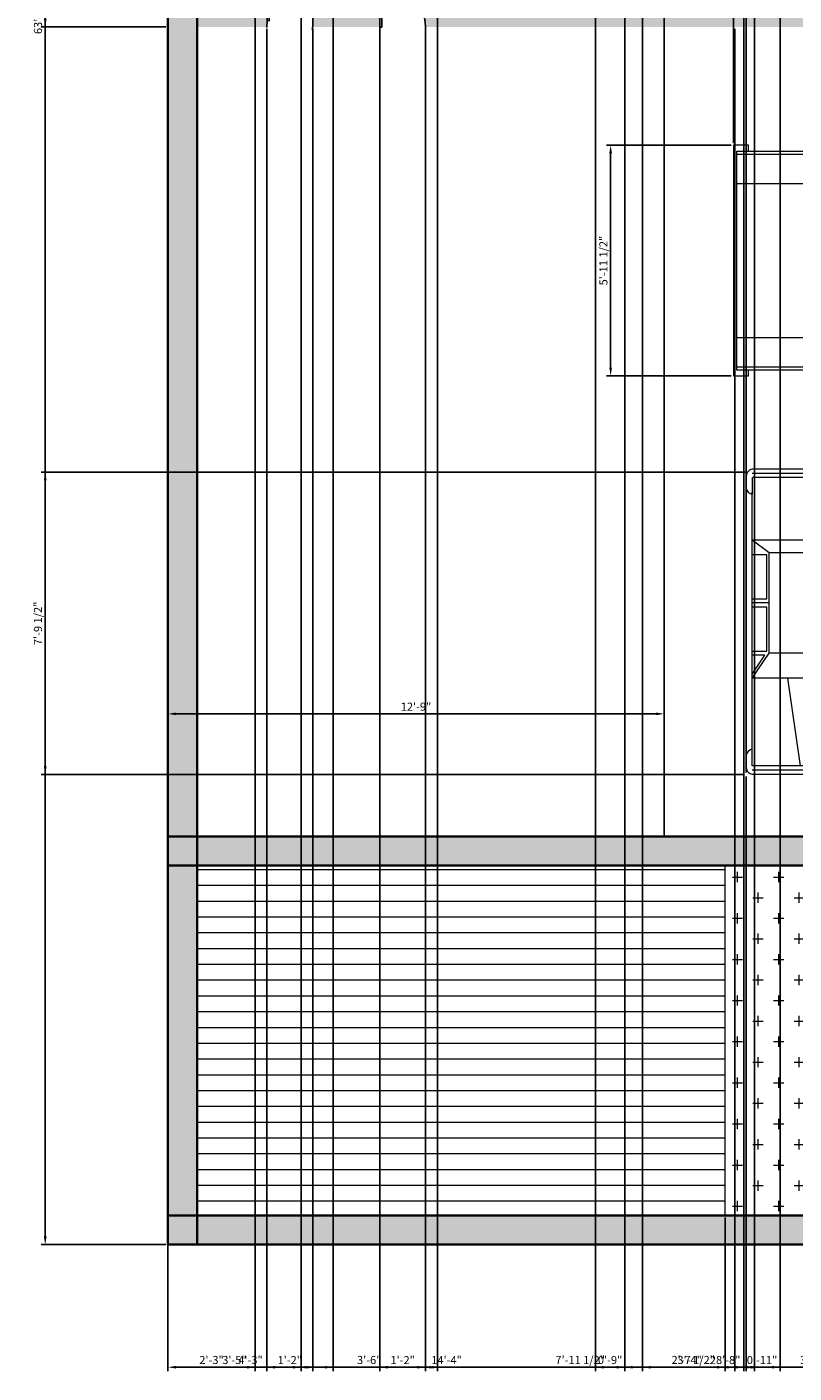
# Model space of a CAD drawing. Units: millimetres. Extents: x 2856 to 3283, y 634 to 1474.
# Tile 1 of 8: x 2856 to 3092, y 634 to 1050. Entities that reach past the tile are written whole.
import ezdxf

# ---------------------------------------------------------------- set-up
doc = ezdxf.new("R2010")
doc.units = ezdxf.units.MM
for name, color, linetype, lineweight in [('A-ANNO-DIMS', 90, 'Continuous', 18), ('A-FLOR', 50, 'Continuous', 18), ('A-FLOR-PATT', 50, 'Continuous', 13), ('A-WALL-PATT', 2, 'Continuous', 13), ('cars', 130, 'Continuous', 13), ('doors', 10, 'Continuous', 25), ('walls', 50, 'Continuous', 35)]:
    doc.layers.add(name, color=color, linetype=linetype, lineweight=lineweight)
doc.styles.get("Standard").update_dxf_attribs({"font": 'arial.ttf'})
doc.dimstyles.new('ISO-25', dxfattribs={"dimtxt": 2.5, "dimasz": 2.5, "dimexe": 1.25, "dimexo": 0.625, "dimtad": 1, "dimdec": 0, "dimlunit": 3, "dimtxsty": 'Standard', "dimcen": 2.5, "dimadec": 0, "dimazin": 0, "dimtfac": 1, "dimtdec": 0, "dimtmove": 0, "dimatfit": 3, "dimfxl": 1, "dimarcsym": 0})

# ---------------------------------------------------------------- blocks, each defined once
blk = doc.blocks.new('*U3')
for p, q in [((0, 0), (0, -6)), ((40, 0), (40, -6))]:
    blk.add_line(p, q)
blk.add_lwpolyline([(0, 0), (0, 40), (1.75, 40), (1.75, 0)], close=True)
blk.add_arc((0, 0), 40, 0, 90)
blk = doc.blocks.new('*U9')
for p, q in [((0.1, -0.41), (0.1, 38.35)), ((2.77, -0.41), (2.77, 38.31)), ((5.44, 42.31), (12.12, 42.31)), ((5.44, -0.41), (5.44, 38.24)), ((5.45, 38.31), (16.12, 38.31)), ((16.12, 38.31), (180.34, 38.31)), ((61.52, -0.41), (61.52, 38.31)), ((61.52, 38.31), (77.54, 27.62)), ((64.19, 38.31), (76.2, 30.29)), ((76.2, 30.29), (76.2, 38.31)), ((78.87, 38.31), (78.87, 28.96)), ((106.91, 28.96), (106.91, 38.31)), ((109.58, 27.62), (109.58, 38.31)), ((112.25, 38.31), (112.25, 28.96)), ((140.29, 28.96), (140.29, 38.31)), ((141.62, 27.62), (149.64, 38.31)), ((149.64, -0.41), (149.64, 38.31)), ((189.69, 38.31), (179.01, 38.31)), ((189.69, 42.31), (183.01, 42.31)), ((189.69, -0.41), (189.69, 38.24)), ((192.36, -0.41), (192.36, 38.31)), ((195.03, -0.41), (195.03, 38.35)), ((77.54, 27.62), (141.62, 27.62)), ((77.54, -0.41), (77.54, 27.62)), ((78.87, 28.96), (106.91, 28.96)), ((112.25, 28.96), (140.29, 28.96)), ((141.62, -0.41), (141.62, 27.62)), ((5.44, 7.6), (61.52, 15.61)), ((0.1, -0.42), (0.1, -39.18)), ((2.77, -0.41), (2.77, -39.13)), ((5.44, -0.42), (5.44, -39.07)), ((5.44, -8.42), (61.52, -16.43)), ((61.52, -0.41), (61.52, -39.13)), ((77.54, -0.41), (77.54, -28.45)), ((141.62, -0.41), (141.62, -28.45)), ((149.64, -0.41), (149.64, -39.13)), ((189.69, -0.42), (189.69, -39.07)), ((192.36, -0.41), (192.36, -39.13)), ((195.03, -0.42), (195.03, -39.18)), ((61.52, -39.13), (77.54, -28.45)), ((64.19, -39.13), (76.2, -31.12)), ((76.2, -31.12), (76.2, -39.13)), ((77.54, -28.45), (141.62, -28.45)), ((78.87, -39.13), (78.87, -29.79)), ((78.87, -29.79), (106.91, -29.79)), ((106.91, -29.79), (106.91, -39.13)), ((109.58, -28.45), (109.58, -39.13)), ((112.25, -29.79), (140.29, -29.79)), ((112.25, -39.13), (112.25, -29.79)), ((140.29, -29.79), (140.29, -39.13)), ((141.62, -28.45), (149.64, -39.13)), ((5.45, -39.13), (16.12, -39.13)), ((16.12, -39.13), (180.34, -39.13)), ((189.69, -39.13), (179.01, -39.13)), ((5.44, -43.14), (12.12, -43.14)), ((189.69, -43.14), (183.01, -43.14))]:
    blk.add_line(p, q)
for centre, radius, start, end in [((5.06, 37.26), 5.06, 85.64554, 168.0943), ((11.45, 37.64), 4.72, 8.13011, 81.86996), ((183.68, 37.64), 4.72, 98.13004, 171.8699), ((190.07, 37.26), 5.06, 11.90574, 94.35446), ((5.06, -38.09), 5.06, 191.9057, 274.3545), ((11.45, -38.46), 4.72, 278.13, 351.8699), ((183.68, -38.46), 4.72, 188.1301, 261.87), ((190.07, -38.09), 5.06, 265.6455, 348.0943)]:
    blk.add_arc(centre, radius, start, end)
blk = doc.blocks.new('*U10')
for p, q in [((1.28, 38.87), (175.66, 38.87)), ((1.28, 28.15), (52.13, 28.15)), ((1.28, -28.15), (52.13, -28.15)), ((1.28, -38.87), (175.66, -38.87))]:
    blk.add_line(p, q)
for points in [[(5.57, 40.01), (5.57, 42.18), (0, 42.18), (0, -42.18), (5.57, -42.18), (5.57, -40.01), (1.28, -40.01), (1.28, 40.01)], [(1.28, 40.01), (175.66, 40.01), (175.66, -40.01), (1.28, -40.01)], [(171.74, 40.01), (175.66, 40.01), (175.66, -40.01), (171.74, -40.01), (171.74, -42.18), (178.14, -42.18), (178.14, 42.18), (171.74, 42.18)], [(71.47, 21.48), (163.42, 21.48), (163.42, -21.48), (71.47, -21.48)]]:
    blk.add_lwpolyline(points, close=True)
for points in [[(57.15, 40.01), (57.15, 32.39), (71.72, 22.83, 0.086577), (72.56, 22.68), (91.59, 22.68, 0.227875), (93.54, 23.62), (97.72, 32.11), (97.72, 40.01)], [(57.15, -40.01), (57.15, -32.39), (71.72, -22.83, -0.086577), (72.56, -22.68), (91.59, -22.68, -0.227875), (93.54, -23.62), (97.72, -32.11), (97.72, -40.01)]]:
    blk.add_lwpolyline(points, format="xyb")
for points in [[(62.08, 30.95), (72.14, 24.35, 0.146139), (72.69, 24.18), (91.42, 24.18, 0.29766), (92.33, 24.78), (95.09, 31.05, 0.541236), (94.86, 31.41), (62.21, 31.41, 0.744989)], [(102.19, 24.58), (106.97, 31, -0.236929), (107.78, 31.41), (162.91, 31.41, -0.621576), (163.11, 31), (158.19, 24.58, -0.233368), (157.39, 24.18), (102.39, 24.18, -0.616908)], [(55.49, 27.42), (68.59, 20.89, -0.284287), (69.14, 19.99), (69.14, -19.99, -0.284287), (68.59, -20.89), (55.49, -27.42, -0.557284), (54.05, -26.53), (54.05, 26.53, -0.557284)], [(171.88, 27.31), (166.83, 24.47, 0.271143), (166.32, 23.6), (166.32, -23.6, 0.271143), (166.83, -24.47), (171.88, -27.31, 0.573387), (173.37, -26.44), (173.37, 26.44, 0.573387)], [(62.08, -30.95), (72.14, -24.35, -0.146139), (72.69, -24.18), (91.42, -24.18, -0.29766), (92.33, -24.78), (95.09, -31.05, -0.541236), (94.86, -31.41), (62.21, -31.41, -0.744989)], [(102.19, -24.58), (106.97, -31, 0.236929), (107.78, -31.41), (162.91, -31.41, 0.621576), (163.11, -31), (158.19, -24.58, 0.233368), (157.39, -24.18), (102.39, -24.18, 0.616908)]]:
    blk.add_lwpolyline(points, format="xyb", close=True)
blk = doc.blocks.new('*D28')
at = {"layer": 'A-ANNO-DIMS', "color": 0, "lineweight": -2, "transparency": 16777216}
for p, q in [((2899.17, 673.31), (2899.17, 634.81)), ((3243.17, 673.31), (3243.17, 634.81)), ((2901.67, 636.06), (3240.67, 636.06))]:
    blk.add_line(p, q, dxfattribs=at)
at = {"layer": 'A-ANNO-DIMS', "color": 0, "transparency": 16777216}
for points in [[(2901.67, 636.48), (2901.67, 635.65), (2899.17, 636.06)], [(3240.67, 636.48), (3240.67, 635.65), (3243.17, 636.06)]]:
    blk.add_solid(points, dxfattribs=at)
at = {"layer": 'Defpoints', "color": 0, "transparency": 16777216}
for p in [(2899.17, 673.94), (3243.17, 673.94), (3243.17, 636.06)]:
    blk.add_point(p, dxfattribs=at)
at = {"layer": 'A-ANNO-DIMS', "color": 0, "transparency": 16777216, "insert": (3071.17, 637.96), "char_height": 2.5, "attachment_point": 5}
blk.add_mtext('28\'-8"', dxfattribs=at)
blk = doc.blocks.new('*D29')
at = {"layer": 'A-ANNO-DIMS', "color": 0, "lineweight": -2, "transparency": 16777216}
for p, q in [((2898.55, 1430.94), (2860.05, 1430.94)), ((2861.3, 676.44), (2861.3, 1428.44)), ((2898.55, 673.94), (2860.05, 673.94))]:
    blk.add_line(p, q, dxfattribs=at)
at = {"layer": 'A-ANNO-DIMS', "color": 0, "transparency": 16777216}
for points in [[(2860.88, 1428.44), (2861.72, 1428.44), (2861.3, 1430.94)], [(2860.88, 676.44), (2861.72, 676.44), (2861.3, 673.94)]]:
    blk.add_solid(points, dxfattribs=at)
at = {"layer": 'Defpoints', "color": 0, "transparency": 16777216}
for p in [(2861.3, 1430.94), (2899.17, 1430.94), (2899.17, 673.94)]:
    blk.add_point(p, dxfattribs=at)
at = {"layer": 'A-ANNO-DIMS', "color": 0, "transparency": 16777216, "insert": (2859.4, 1052.44), "char_height": 2.5, "attachment_point": 5, "rotation": 90}
blk.add_mtext('63\'-1"', dxfattribs=at)
blk = doc.blocks.new('*D32')
at = {"layer": 'A-ANNO-DIMS', "color": 0, "lineweight": -2, "transparency": 16777216}
for p, q in [((3071.17, 682.31), (3071.17, 634.81)), ((2899.17, 673.31), (2899.17, 634.81)), ((2901.67, 636.06), (3068.67, 636.06))]:
    blk.add_line(p, q, dxfattribs=at)
at = {"layer": 'A-ANNO-DIMS', "color": 0, "transparency": 16777216}
for points in [[(2901.67, 636.48), (2901.67, 635.65), (2899.17, 636.06)], [(3068.67, 636.48), (3068.67, 635.65), (3071.17, 636.06)]]:
    blk.add_solid(points, dxfattribs=at)
at = {"layer": 'Defpoints', "color": 0, "transparency": 16777216}
for p in [(3071.17, 682.94), (2899.17, 673.94), (3071.17, 636.06)]:
    blk.add_point(p, dxfattribs=at)
at = {"layer": 'A-ANNO-DIMS', "color": 0, "transparency": 16777216, "insert": (2985.17, 637.94), "char_height": 2.5, "attachment_point": 5}
blk.add_mtext('14\'-4"', dxfattribs=at)
blk = doc.blocks.new('*D33')
at = {"layer": 'A-ANNO-DIMS', "color": 0, "lineweight": -2, "transparency": 16777216}
for p, q in [((3073.7, 1014.05), (3073.7, 1470.06)), ((3076.2, 1468.81), (3221.68, 1468.81)), ((3224.18, 1014.05), (3224.18, 1470.06))]:
    blk.add_line(p, q, dxfattribs=at)
at = {"layer": 'A-ANNO-DIMS', "color": 0, "transparency": 16777216}
for points in [[(3076.2, 1469.23), (3076.2, 1468.4), (3073.7, 1468.81)], [(3221.68, 1469.23), (3221.68, 1468.4), (3224.18, 1468.81)]]:
    blk.add_solid(points, dxfattribs=at)
at = {"layer": 'Defpoints', "color": 0, "transparency": 16777216}
for p in [(3224.18, 1468.81), (3073.7, 1013.42), (3224.18, 1013.42)]:
    blk.add_point(p, dxfattribs=at)
at = {"layer": 'A-ANNO-DIMS', "color": 0, "transparency": 16777216, "insert": (3148.94, 1470.73), "char_height": 2.5, "attachment_point": 5}
blk.add_mtext('12\'-6 1/2"', dxfattribs=at)
blk = doc.blocks.new('*D34')
at = {"layer": 'A-ANNO-DIMS', "color": 0, "lineweight": -2, "transparency": 16777216}
for p, q in [((3073.07, 1013.42), (3034.57, 1013.42)), ((3035.82, 944.67), (3035.82, 1010.92)), ((3073.07, 942.17), (3034.57, 942.17))]:
    blk.add_line(p, q, dxfattribs=at)
at = {"layer": 'A-ANNO-DIMS', "color": 0, "transparency": 16777216}
for points in [[(3035.41, 1010.92), (3036.24, 1010.92), (3035.82, 1013.42)], [(3035.41, 944.67), (3036.24, 944.67), (3035.82, 942.17)]]:
    blk.add_solid(points, dxfattribs=at)
at = {"layer": 'Defpoints', "color": 0, "transparency": 16777216}
for p in [(3035.82, 1013.42), (3073.7, 1013.42), (3073.7, 942.17)]:
    blk.add_point(p, dxfattribs=at)
at = {"layer": 'A-ANNO-DIMS', "color": 0, "transparency": 16777216, "insert": (3033.91, 977.79), "char_height": 2.5, "attachment_point": 5, "rotation": 90}
blk.add_mtext('5\'-11 1/2"', dxfattribs=at)
blk = doc.blocks.new('*D35')
at = {"layer": 'A-ANNO-DIMS', "color": 0, "lineweight": -2, "transparency": 16777216}
for p, q in [((3077.47, 912.44), (2860.05, 912.44)), ((2861.3, 821.59), (2861.3, 909.94)), ((3077.06, 819.09), (2860.05, 819.09))]:
    blk.add_line(p, q, dxfattribs=at)
at = {"layer": 'A-ANNO-DIMS', "color": 0, "transparency": 16777216}
for points in [[(2860.88, 909.94), (2861.72, 909.94), (2861.3, 912.44)], [(2860.88, 821.59), (2861.72, 821.59), (2861.3, 819.09)]]:
    blk.add_solid(points, dxfattribs=at)
at = {"layer": 'Defpoints', "color": 0, "transparency": 16777216}
for p in [(2861.3, 912.44), (3078.1, 912.44), (3077.68, 819.09)]:
    blk.add_point(p, dxfattribs=at)
at = {"layer": 'A-ANNO-DIMS', "color": 0, "transparency": 16777216, "insert": (2859.38, 865.77), "char_height": 2.5, "attachment_point": 5, "rotation": 90}
blk.add_mtext('7\'-9 1/2"', dxfattribs=at)
blk = doc.blocks.new('*D36')
at = {"layer": 'A-ANNO-DIMS', "color": 0, "lineweight": -2, "transparency": 16777216}
for p, q in [((3077.68, 818.47), (3077.68, 634.81)), ((3118.46, 818.47), (3118.46, 634.81)), ((3080.18, 636.06), (3115.96, 636.06))]:
    blk.add_line(p, q, dxfattribs=at)
at = {"layer": 'A-ANNO-DIMS', "color": 0, "transparency": 16777216}
for points in [[(3080.18, 636.48), (3080.18, 635.65), (3077.68, 636.06)], [(3115.96, 636.48), (3115.96, 635.65), (3118.46, 636.06)]]:
    blk.add_solid(points, dxfattribs=at)
at = {"layer": 'Defpoints', "color": 0, "transparency": 16777216}
for p in [(3077.68, 819.09), (3118.46, 819.09), (3118.46, 636.06)]:
    blk.add_point(p, dxfattribs=at)
at = {"layer": 'A-ANNO-DIMS', "color": 0, "transparency": 16777216, "insert": (3098.07, 637.97), "char_height": 2.5, "attachment_point": 5}
blk.add_mtext('3\'-5"', dxfattribs=at)
blk = doc.blocks.new('*D39')
at = {"layer": 'A-ANNO-DIMS', "color": 0, "lineweight": -2, "transparency": 16777216}
for p, q in [((2899.17, 800.56), (2899.17, 839.06)), ((2901.67, 837.81), (3049.84, 837.81)), ((3052.34, 800.56), (3052.34, 839.06))]:
    blk.add_line(p, q, dxfattribs=at)
at = {"layer": 'A-ANNO-DIMS', "color": 0, "transparency": 16777216}
for points in [[(2901.67, 838.23), (2901.67, 837.4), (2899.17, 837.81)], [(3049.84, 838.23), (3049.84, 837.4), (3052.34, 837.81)]]:
    blk.add_solid(points, dxfattribs=at)
at = {"layer": 'Defpoints', "color": 0, "transparency": 16777216}
for p in [(3052.34, 837.81), (2899.17, 799.94), (3052.34, 799.94)]:
    blk.add_point(p, dxfattribs=at)
at = {"layer": 'A-ANNO-DIMS', "color": 0, "transparency": 16777216, "insert": (2975.76, 839.71), "char_height": 2.5, "attachment_point": 5}
blk.add_mtext('12\'-9"', dxfattribs=at)
blk = doc.blocks.new('*D43')
at = {"layer": 'A-ANNO-DIMS', "color": 0, "lineweight": -2, "transparency": 16777216}
for p, q in [((3052.34, 800.56), (3052.34, 1470.06)), ((3054.84, 1468.81), (3075.18, 1468.81)), ((3077.68, 819.72), (3077.68, 1470.06))]:
    blk.add_line(p, q, dxfattribs=at)
at = {"layer": 'A-ANNO-DIMS', "color": 0, "transparency": 16777216}
for points in [[(3054.84, 1469.23), (3054.84, 1468.4), (3052.34, 1468.81)], [(3075.18, 1469.23), (3075.18, 1468.4), (3077.68, 1468.81)]]:
    blk.add_solid(points, dxfattribs=at)
at = {"layer": 'Defpoints', "color": 0, "transparency": 16777216}
for p in [(3077.68, 1468.81), (3077.68, 819.09), (3052.34, 799.94)]:
    blk.add_point(p, dxfattribs=at)
at = {"layer": 'A-ANNO-DIMS', "color": 0, "transparency": 16777216, "insert": (3065.01, 1470.73), "char_height": 2.5, "attachment_point": 5}
blk.add_mtext('2\'-1 1/2"', dxfattribs=at)
blk = doc.blocks.new('*D58')
at = {"layer": 'A-ANNO-DIMS', "color": 0, "lineweight": -2, "transparency": 16777216}
for p, q in [((2950.17, 1116.31), (2950.17, 634.81)), ((2899.17, 1107.31), (2899.17, 634.81)), ((2901.67, 636.06), (2947.67, 636.06))]:
    blk.add_line(p, q, dxfattribs=at)
at = {"layer": 'A-ANNO-DIMS', "color": 0, "transparency": 16777216}
for points in [[(2901.67, 636.48), (2901.67, 635.65), (2899.17, 636.06)], [(2947.67, 636.48), (2947.67, 635.65), (2950.17, 636.06)]]:
    blk.add_solid(points, dxfattribs=at)
at = {"layer": 'Defpoints', "color": 0, "transparency": 16777216}
for p in [(2950.17, 1116.94), (2899.17, 1107.94), (2950.17, 636.06)]:
    blk.add_point(p, dxfattribs=at)
at = {"layer": 'A-ANNO-DIMS', "color": 0, "transparency": 16777216, "insert": (2924.67, 637.97), "char_height": 2.5, "attachment_point": 5}
blk.add_mtext('4\'-3"', dxfattribs=at)
blk = doc.blocks.new('*D60')
at = {"layer": 'A-ANNO-DIMS', "color": 0, "lineweight": -2, "transparency": 16777216}
for p, q in [((2898.55, 1116.94), (2860.05, 1116.94)), ((2861.3, 1052.44), (2861.3, 1114.44)), ((2898.55, 1049.94), (2860.05, 1049.94))]:
    blk.add_line(p, q, dxfattribs=at)
at = {"layer": 'A-ANNO-DIMS', "color": 0, "transparency": 16777216}
for points in [[(2860.88, 1114.44), (2861.72, 1114.44), (2861.3, 1116.94)], [(2860.88, 1052.44), (2861.72, 1052.44), (2861.3, 1049.94)]]:
    blk.add_solid(points, dxfattribs=at)
at = {"layer": 'Defpoints', "color": 0, "transparency": 16777216}
for p in [(2861.3, 1116.94), (2899.17, 1116.94), (2899.17, 1049.94)]:
    blk.add_point(p, dxfattribs=at)
at = {"layer": 'A-ANNO-DIMS', "color": 0, "transparency": 16777216, "insert": (2859.4, 1083.44), "char_height": 2.5, "attachment_point": 5, "rotation": 90}
blk.add_mtext('5\'-7"', dxfattribs=at)
blk = doc.blocks.new('*D61')
at = {"layer": 'A-ANNO-DIMS', "color": 0, "lineweight": -2, "transparency": 16777216}
for p, q in [((3031.17, 1430.31), (3031.17, 634.81)), ((3040.17, 1430.31), (3040.17, 634.81)), ((3033.67, 636.06), (3037.67, 636.06))]:
    blk.add_line(p, q, dxfattribs=at)
at = {"layer": 'A-ANNO-DIMS', "color": 0, "transparency": 16777216}
for points in [[(3033.67, 636.48), (3033.67, 635.65), (3031.17, 636.06)], [(3037.67, 636.48), (3037.67, 635.65), (3040.17, 636.06)]]:
    blk.add_solid(points, dxfattribs=at)
at = {"layer": 'Defpoints', "color": 0, "transparency": 16777216}
for p in [(3031.17, 1430.94), (3040.17, 1430.94), (3040.17, 636.06)]:
    blk.add_point(p, dxfattribs=at)
at = {"layer": 'A-ANNO-DIMS', "color": 0, "transparency": 16777216, "insert": (3035.67, 637.96), "char_height": 2.5, "attachment_point": 5}
blk.add_mtext('0\'-9"', dxfattribs=at)
blk = doc.blocks.new('*D66')
at = {"layer": 'A-ANNO-DIMS', "color": 0, "lineweight": -2, "transparency": 16777216}
for p, q in [((2929.71, 1049.31), (2929.71, 634.81)), ((2943.86, 1049.31), (2943.86, 634.81)), ((2932.21, 636.06), (2941.36, 636.06))]:
    blk.add_line(p, q, dxfattribs=at)
at = {"layer": 'A-ANNO-DIMS', "color": 0, "transparency": 16777216}
for points in [[(2932.21, 636.48), (2932.21, 635.65), (2929.71, 636.06)], [(2941.36, 636.48), (2941.36, 635.65), (2943.86, 636.06)]]:
    blk.add_solid(points, dxfattribs=at)
at = {"layer": 'Defpoints', "color": 0, "transparency": 16777216}
for p in [(2929.71, 1049.94), (2943.86, 1049.94), (2943.86, 636.06)]:
    blk.add_point(p, dxfattribs=at)
at = {"layer": 'A-ANNO-DIMS', "color": 0, "transparency": 16777216, "insert": (2936.79, 637.94), "char_height": 2.5, "attachment_point": 5}
blk.add_mtext('1\'-2"', dxfattribs=at)
blk = doc.blocks.new('*D67')
at = {"layer": 'A-ANNO-DIMS', "color": 0, "lineweight": -2, "transparency": 16777216}
for p, q in [((2964.56, 1049.25), (2964.56, 634.81)), ((2978.69, 1049.31), (2978.69, 634.81)), ((2967.06, 636.06), (2976.19, 636.06))]:
    blk.add_line(p, q, dxfattribs=at)
at = {"layer": 'A-ANNO-DIMS', "color": 0, "transparency": 16777216}
for points in [[(2967.06, 636.48), (2967.06, 635.65), (2964.56, 636.06)], [(2976.19, 636.48), (2976.19, 635.65), (2978.69, 636.06)]]:
    blk.add_solid(points, dxfattribs=at)
at = {"layer": 'Defpoints', "color": 0, "transparency": 16777216}
for p in [(2964.56, 1049.87), (2978.69, 1049.94), (2978.69, 636.06)]:
    blk.add_point(p, dxfattribs=at)
at = {"layer": 'A-ANNO-DIMS', "color": 0, "transparency": 16777216, "insert": (2971.63, 637.94), "char_height": 2.5, "attachment_point": 5}
blk.add_mtext('1\'-2"', dxfattribs=at)
blk = doc.blocks.new('*D69')
at = {"layer": 'A-ANNO-DIMS', "color": 0, "lineweight": -2, "transparency": 16777216}
for p, q in [((2940.27, 1421.31), (2940.27, 634.81)), ((2982.35, 1421.31), (2982.35, 634.81)), ((2942.77, 636.06), (2979.85, 636.06))]:
    blk.add_line(p, q, dxfattribs=at)
at = {"layer": 'A-ANNO-DIMS', "color": 0, "transparency": 16777216}
for points in [[(2942.77, 636.48), (2942.77, 635.65), (2940.27, 636.06)], [(2979.85, 636.48), (2979.85, 635.65), (2982.35, 636.06)]]:
    blk.add_solid(points, dxfattribs=at)
at = {"layer": 'Defpoints', "color": 0, "transparency": 16777216}
for p in [(2940.27, 1421.94), (2982.35, 1421.94), (2982.35, 636.06)]:
    blk.add_point(p, dxfattribs=at)
at = {"layer": 'A-ANNO-DIMS', "color": 0, "transparency": 16777216, "insert": (2961.31, 637.97), "char_height": 2.5, "attachment_point": 5}
blk.add_mtext('3\'-6"', dxfattribs=at)
blk = doc.blocks.new('*D70')
at = {"layer": 'A-ANNO-DIMS', "color": 0, "lineweight": -2, "transparency": 16777216}
for p, q in [((3045.69, 1421.31), (3045.69, 634.81)), ((3076.97, 1421.31), (3076.97, 634.81)), ((3048.19, 636.06), (3074.47, 636.06))]:
    blk.add_line(p, q, dxfattribs=at)
at = {"layer": 'A-ANNO-DIMS', "color": 0, "transparency": 16777216}
for points in [[(3048.19, 636.48), (3048.19, 635.65), (3045.69, 636.06)], [(3074.47, 636.48), (3074.47, 635.65), (3076.97, 636.06)]]:
    blk.add_solid(points, dxfattribs=at)
at = {"layer": 'Defpoints', "color": 0, "transparency": 16777216}
for p in [(3045.69, 1421.94), (3076.97, 1421.94), (3076.97, 636.06)]:
    blk.add_point(p, dxfattribs=at)
at = {"layer": 'A-ANNO-DIMS', "color": 0, "transparency": 16777216, "insert": (3061.33, 637.98), "char_height": 2.5, "attachment_point": 5}
blk.add_mtext('2\'-7 1/2"', dxfattribs=at)
blk = doc.blocks.new('*D76')
at = {"layer": 'A-ANNO-DIMS', "color": 0, "lineweight": -2, "transparency": 16777216}
for p, q in [((2899.17, 1421.31), (2899.17, 634.81)), ((2940.27, 1421.31), (2940.27, 634.81)), ((2901.67, 636.06), (2937.77, 636.06))]:
    blk.add_line(p, q, dxfattribs=at)
at = {"layer": 'A-ANNO-DIMS', "color": 0, "transparency": 16777216}
for points in [[(2901.67, 636.48), (2901.67, 635.65), (2899.17, 636.06)], [(2937.77, 636.48), (2937.77, 635.65), (2940.27, 636.06)]]:
    blk.add_solid(points, dxfattribs=at)
at = {"layer": 'Defpoints', "color": 0, "transparency": 16777216}
for p in [(2899.17, 1421.94), (2940.27, 1421.94), (2940.27, 636.06)]:
    blk.add_point(p, dxfattribs=at)
at = {"layer": 'A-ANNO-DIMS', "color": 0, "transparency": 16777216, "insert": (2919.72, 637.97), "char_height": 2.5, "attachment_point": 5}
blk.add_mtext('3\'-5"', dxfattribs=at)
blk = doc.blocks.new('*D87')
at = {"layer": 'A-ANNO-DIMS', "color": 0, "lineweight": -2, "transparency": 16777216}
for p, q in [((2978.69, 1049.31), (2978.69, 634.81)), ((3074.17, 1049.31), (3074.17, 634.81)), ((2981.19, 636.06), (3071.67, 636.06))]:
    blk.add_line(p, q, dxfattribs=at)
at = {"layer": 'A-ANNO-DIMS', "color": 0, "transparency": 16777216}
for points in [[(2981.19, 636.48), (2981.19, 635.65), (2978.69, 636.06)], [(3071.67, 636.48), (3071.67, 635.65), (3074.17, 636.06)]]:
    blk.add_solid(points, dxfattribs=at)
at = {"layer": 'Defpoints', "color": 0, "transparency": 16777216}
for p in [(2978.69, 1049.94), (3074.17, 1049.94), (3074.17, 636.06)]:
    blk.add_point(p, dxfattribs=at)
at = {"layer": 'A-ANNO-DIMS', "color": 0, "transparency": 16777216, "insert": (3026.43, 637.98), "char_height": 2.5, "attachment_point": 5}
blk.add_mtext('7\'-11 1/2"', dxfattribs=at)
blk = doc.blocks.new('*D90')
at = {"layer": 'A-ANNO-DIMS', "color": 0, "lineweight": -2, "transparency": 16777216}
for p, q in [((2899.17, 1421.31), (2899.17, 634.81)), ((2926.08, 1404.73), (2926.08, 634.81)), ((2901.67, 636.06), (2923.58, 636.06))]:
    blk.add_line(p, q, dxfattribs=at)
at = {"layer": 'A-ANNO-DIMS', "color": 0, "transparency": 16777216}
for points in [[(2901.67, 636.48), (2901.67, 635.65), (2899.17, 636.06)], [(2923.58, 636.48), (2923.58, 635.65), (2926.08, 636.06)]]:
    blk.add_solid(points, dxfattribs=at)
at = {"layer": 'Defpoints', "color": 0, "transparency": 16777216}
for p in [(2899.17, 1421.94), (2926.08, 1405.35), (2926.08, 636.06)]:
    blk.add_point(p, dxfattribs=at)
at = {"layer": 'A-ANNO-DIMS', "color": 0, "transparency": 16777216, "insert": (2912.63, 637.97), "char_height": 2.5, "attachment_point": 5}
blk.add_mtext('2\'-3"', dxfattribs=at)
blk = doc.blocks.new('*D94')
at = {"layer": 'A-ANNO-DIMS', "color": 0, "lineweight": -2, "transparency": 16777216}
for p, q in [((3040.17, 1287.31), (3040.17, 634.81)), ((3080.25, 1257.69), (3080.25, 634.81)), ((3042.67, 636.06), (3077.75, 636.06))]:
    blk.add_line(p, q, dxfattribs=at)
at = {"layer": 'A-ANNO-DIMS', "color": 0, "transparency": 16777216}
for points in [[(3042.67, 636.48), (3042.67, 635.65), (3040.17, 636.06)], [(3077.75, 636.48), (3077.75, 635.65), (3080.25, 636.06)]]:
    blk.add_solid(points, dxfattribs=at)
at = {"layer": 'Defpoints', "color": 0, "transparency": 16777216}
for p in [(3040.17, 1287.94), (3080.25, 1258.32), (3080.25, 636.06)]:
    blk.add_point(p, dxfattribs=at)
at = {"layer": 'A-ANNO-DIMS', "color": 0, "transparency": 16777216, "insert": (3060.21, 637.97), "char_height": 2.5, "attachment_point": 5}
blk.add_mtext('3\'-4"', dxfattribs=at)
blk = doc.blocks.new('*D98')
at = {"layer": 'A-ANNO-DIMS', "color": 0, "lineweight": -2, "transparency": 16777216}
for p, q in [((3088.17, 1430.31), (3088.17, 634.81)), ((3076.97, 1421.31), (3076.97, 634.81)), ((3079.47, 636.06), (3085.67, 636.06))]:
    blk.add_line(p, q, dxfattribs=at)
at = {"layer": 'A-ANNO-DIMS', "color": 0, "transparency": 16777216}
for points in [[(3079.47, 636.48), (3079.47, 635.65), (3076.97, 636.06)], [(3085.67, 636.48), (3085.67, 635.65), (3088.17, 636.06)]]:
    blk.add_solid(points, dxfattribs=at)
at = {"layer": 'Defpoints', "color": 0, "transparency": 16777216}
for p in [(3088.17, 1430.94), (3076.97, 1421.94), (3088.17, 636.06)]:
    blk.add_point(p, dxfattribs=at)
at = {"layer": 'A-ANNO-DIMS', "color": 0, "transparency": 16777216, "insert": (3082.57, 637.96), "char_height": 2.5, "attachment_point": 5}
blk.add_mtext('0\'-11"', dxfattribs=at)

msp = doc.modelspace()

# ---------------------------------------------------------------- hatches: boundary and pattern name
at = {"layer": 'A-FLOR-PATT'}
h = msp.add_hatch(dxfattribs=at)
h.set_pattern_fill('ANSI31', color=256, scale=1.53546, angle=-45, style=0)
h.paths.add_polyline_path([(2908.17, 682.94), (3071.17, 682.94), (3071.17, 790.94), (2908.17, 790.94)])
h = msp.add_hatch(dxfattribs=at)
h.set_pattern_fill('CROSS', color=256)
h.paths.add_polyline_path([(3234.17, 790.94), (3071.17, 790.94), (3071.17, 682.94), (3234.17, 682.94)])
at = {"layer": 'A-WALL-PATT'}
h = msp.add_hatch(color=256, dxfattribs=at)
h.dxf.hatch_style = 1
h.paths.add_polyline_path([(2908.17, 1430.94), (2899.17, 1430.94), (2899.17, 1421.94), (2908.17, 1421.94)])
h.paths.add_polyline_path([(2908.17, 1421.94), (2899.17, 1421.94), (2899.17, 1296.94), (2908.17, 1296.94)])
h.paths.add_polyline_path([(2940.27, 1430.94), (2908.17, 1430.94), (2908.17, 1421.94), (2940.27, 1421.94)])
h.paths.add_polyline_path([(3031.17, 1430.94), (2982.35, 1430.94), (2982.35, 1421.94), (3031.17, 1421.94)])
h.paths.add_polyline_path([(3150.5, 1430.94), (3097.17, 1430.94), (3097.17, 1421.94), (3150.5, 1421.94)])
h.paths.add_polyline_path([(3097.17, 1430.94), (3088.17, 1430.94), (3088.17, 1421.94), (3097.17, 1421.94)])
h.paths.add_polyline_path([(3097.17, 1421.94), (3088.17, 1421.94), (3088.17, 1337.94), (3097.17, 1337.94)])
h.paths.add_polyline_path([(3088.17, 1337.94), (3040.17, 1337.94), (3040.17, 1328.94), (3088.17, 1328.94)])
h.paths.add_polyline_path([(3097.17, 1337.94), (3088.17, 1337.94), (3088.17, 1328.94), (3097.17, 1328.94)])
h.paths.add_polyline_path([(3097.17, 1328.94), (3088.17, 1328.94), (3088.17, 1296.94), (3097.17, 1296.94)])
h.paths.add_polyline_path([(3097.17, 1296.94), (3088.17, 1296.94), (3088.17, 1287.94), (3097.17, 1287.94)])
h.paths.add_polyline_path([(3040.17, 1421.94), (3031.17, 1421.94), (3031.17, 1337.94), (3040.17, 1337.94)])
h.paths.add_polyline_path([(3040.17, 1337.94), (3031.17, 1337.94), (3031.17, 1328.94), (3040.17, 1328.94)])
h.paths.add_polyline_path([(3040.17, 1430.94), (3031.17, 1430.94), (3031.17, 1421.94), (3040.17, 1421.94)])
h.paths.add_polyline_path([(3243.17, 1421.94), (3234.17, 1421.94), (3234.17, 1385.21), (3243.17, 1385.21)])
h.paths.add_polyline_path([(3243.17, 1430.94), (3234.17, 1430.94), (3234.17, 1421.94), (3243.17, 1421.94)])
h.paths.add_polyline_path([(3234.17, 1430.94), (3189.65, 1430.94), (3189.65, 1421.94), (3234.17, 1421.94)])
h.paths.add_polyline_path([(3243.17, 1345.16), (3234.17, 1345.16), (3234.17, 1296.94), (3243.17, 1296.94)])
h.paths.add_polyline_path([(3234.17, 1296.94), (3128.45, 1296.94, -0.06768), (3129.44, 1289.59), (3129.44, 1287.94), (3234.17, 1287.94)])
h.paths.add_polyline_path([(3031.17, 1296.94), (2908.17, 1296.94), (2908.17, 1287.94), (3031.17, 1287.94)])
h.paths.add_polyline_path([(3040.17, 1296.94), (3031.17, 1296.94), (3031.17, 1287.94), (3040.17, 1287.94)])
h.paths.add_polyline_path([(2908.17, 1296.94), (2899.17, 1296.94), (2899.17, 1287.94), (2908.17, 1287.94)])
h.paths.add_polyline_path([(2908.17, 1287.94), (2899.17, 1287.94), (2899.17, 1235.12), (2908.17, 1235.12)])
h.paths.add_polyline_path([(3040.17, 1287.94), (3031.17, 1287.94), (3031.17, 1165.94), (3040.17, 1165.94)])
h.paths.add_polyline_path([(3165.17, 1165.94), (3040.17, 1165.94), (3040.17, 1156.94), (3165.17, 1156.94)])
h.paths.add_polyline_path([(3040.17, 1165.94), (3031.17, 1165.94), (3031.17, 1156.94), (3040.17, 1156.94)])
h.paths.add_polyline_path([(3040.17, 1156.94), (3031.17, 1156.94), (3031.17, 1147.75, -0.068303), (3038.59, 1148.77), (3040.17, 1148.77)])
h.paths.add_polyline_path([(3174.17, 1197.55), (3166.11, 1197.55), (3165.17, 1197.55), (3165.17, 1165.94), (3174.17, 1165.94)])
h.paths.add_polyline_path([(3174.17, 1165.94), (3165.17, 1165.94), (3165.17, 1156.94), (3174.17, 1156.94)])
h.paths.add_polyline_path([(3234.17, 1165.94), (3174.17, 1165.94), (3174.17, 1156.94), (3234.17, 1156.94)])
h.paths.add_polyline_path([(3243.17, 1165.94), (3234.17, 1165.94), (3234.17, 1156.94), (3243.17, 1156.94)])
h.paths.add_polyline_path([(3243.17, 1172.31), (3234.17, 1172.31), (3234.17, 1165.94), (3243.17, 1165.94)])
h.paths.add_polyline_path([(3243.17, 1222.94), (3234.17, 1222.94), (3234.17, 1213.94), (3243.17, 1213.94)])
h.paths.add_polyline_path([(3234.17, 1222.94), (3174.17, 1222.94), (3174.17, 1213.94), (3234.17, 1213.94)])
h.paths.add_polyline_path([(3174.17, 1222.94), (3165.17, 1222.94), (3165.17, 1213.94), (3174.17, 1213.94)])
h.paths.add_polyline_path([(3174.17, 1270.54, -0.139319), (3166.75, 1268.43), (3165.17, 1268.43), (3165.17, 1222.94), (3174.17, 1222.94)])
h.paths.add_polyline_path([(3243.17, 1243.94), (3234.17, 1243.94), (3234.17, 1222.94), (3243.17, 1222.94)])
h.paths.add_polyline_path([(3243.17, 1213.94), (3234.17, 1213.94), (3234.17, 1203.68), (3243.17, 1203.68)])
h.paths.add_polyline_path([(3174.17, 1213.94), (3165.17, 1213.94), (3165.17, 1210.62), (3166.11, 1210.62, -0.16772), (3174.17, 1207.84)])
h.paths.add_polyline_path([(3243.17, 1296.94), (3234.17, 1296.94), (3234.17, 1287.94), (3243.17, 1287.94)])
h.paths.add_polyline_path([(3243.17, 1287.94), (3234.17, 1287.94), (3234.17, 1276.76), (3243.17, 1276.76)])
h.paths.add_polyline_path([(3174.17, 1287.94), (3165.17, 1287.94), (3165.17, 1282.56), (3166.75, 1282.56), (3174.17, 1282.56)])
h.paths.add_polyline_path([(2908.17, 1190.69), (2899.17, 1190.69), (2899.17, 1116.94), (2908.17, 1116.94)])
h.paths.add_polyline_path([(2908.17, 1107.94), (2899.17, 1107.94), (2899.17, 1058.94), (2908.17, 1058.94)])
h.paths.add_polyline_path([(2908.17, 1116.94), (2899.17, 1116.94), (2899.17, 1107.94), (2908.17, 1107.94)])
h.paths.add_polyline_path([(2959.17, 1107.94), (2950.17, 1107.94), (2950.17, 1058.94), (2959.17, 1058.94)])
h.paths.add_polyline_path([(2959.17, 1116.94), (2950.17, 1116.94), (2950.17, 1107.94), (2959.17, 1107.94)])
h.paths.add_polyline_path([(2950.17, 1116.94), (2908.17, 1116.94), (2908.17, 1107.94), (2950.17, 1107.94)])
h.paths.add_polyline_path([(3031.17, 1116.94), (2959.17, 1116.94), (2959.17, 1107.94), (3031.17, 1107.94)])
h.paths.add_polyline_path([(3074.17, 1116.94), (3065.17, 1116.94), (3065.17, 1107.94), (3074.17, 1107.94)])
h.paths.add_polyline_path([(3065.17, 1116.94), (3040.17, 1116.94), (3040.17, 1107.94), (3065.17, 1107.94)])
h.paths.add_polyline_path([(3040.17, 1116.94), (3031.17, 1116.94), (3031.17, 1107.94), (3040.17, 1107.94)])
h.paths.add_polyline_path([(3040.17, 1121.26), (3038.59, 1121.26), (3031.17, 1121.26), (3031.17, 1116.94), (3040.17, 1116.94)])
h.paths.add_polyline_path([(3074.17, 1107.94), (3065.17, 1107.94), (3065.17, 1058.94), (3074.17, 1058.94)])
h.paths.add_polyline_path([(3074.17, 1058.94), (3065.17, 1058.94), (3065.17, 1049.94), (3074.17, 1049.94)])
h.paths.add_polyline_path([(3065.17, 1058.94), (2975.4, 1058.94, -0.174756), (2978.69, 1049.94), (3065.17, 1049.94)])
h.paths.add_polyline_path([(2929.83, 1051.89), (2930.25, 1058.94), (2908.17, 1058.94), (2908.17, 1049.94), (2929.71, 1049.94)])
h.paths.add_polyline_path([(2908.17, 1058.94), (2899.17, 1058.94), (2899.17, 1049.94), (2908.17, 1049.94)])
h.paths.add_polyline_path([(2950.17, 1058.94), (2942.07, 1058.94, -0.146602), (2943.93, 1051.05), (2943.86, 1049.94), (2950.17, 1049.94)])
h.paths.add_polyline_path([(2959.17, 1058.94), (2950.17, 1058.94), (2950.17, 1049.94), (2959.17, 1049.94)])
h.paths.add_polyline_path([(2964.56, 1058.94), (2959.17, 1058.94), (2959.17, 1049.94), (2964.56, 1049.94)])
h.paths.add_polyline_path([(2908.17, 1049.94), (2899.17, 1049.94), (2899.17, 799.94), (2908.17, 799.94)])
h.paths.add_polyline_path([(3234.17, 1058.94), (3074.17, 1058.94), (3074.17, 1049.94), (3234.17, 1049.94)])
h.paths.add_polyline_path([(3243.17, 1156.94), (3234.17, 1156.94), (3234.17, 1058.94), (3243.17, 1058.94)])
h.paths.add_polyline_path([(3243.17, 1058.94), (3234.17, 1058.94), (3234.17, 1049.94), (3243.17, 1049.94)])
h.paths.add_polyline_path([(3243.17, 1049.94), (3234.17, 1049.94), (3234.17, 931.7), (3234.17, 799.94), (3243.17, 799.94), (3243.17, 931.7)])
h.paths.add_polyline_path([(2908.17, 790.94), (2899.17, 790.94), (2899.17, 682.94), (2908.17, 682.94)])
h.paths.add_polyline_path([(2908.17, 799.94), (2899.17, 799.94), (2899.17, 790.94), (2908.17, 790.94)])
h.paths.add_polyline_path([(3234.17, 799.94), (2908.17, 799.94), (2908.17, 790.94), (3234.17, 790.94)])
h.paths.add_polyline_path([(3243.17, 799.94), (3234.17, 799.94), (3234.17, 790.94), (3243.17, 790.94)])
h.paths.add_polyline_path([(3243.17, 790.94), (3234.17, 790.94), (3234.17, 682.94), (3243.17, 682.94)])
h.paths.add_polyline_path([(3234.17, 682.94), (2908.17, 682.94), (2908.17, 673.94), (3234.17, 673.94)])
h.paths.add_polyline_path([(3243.17, 682.94), (3234.17, 682.94), (3234.17, 673.94), (3243.17, 673.94)])
h.paths.add_polyline_path([(2908.17, 682.94), (2899.17, 682.94), (2899.17, 673.94), (2908.17, 673.94)])

# ---------------------------------------------------------------- linework, layer by layer
at = {"layer": 'A-FLOR'}
for p, q in [((3052.34, 1049.94), (3052.34, 799.94)), ((3071.17, 682.94), (3071.17, 790.94))]:
    msp.add_line(p, q, dxfattribs=at)
at = {"layer": 'walls'}
for p, q in [((2899.17, 1430.94), (2899.17, 790.94)), ((2908.17, 1430.94), (2908.17, 790.94)), ((3243.17, 799.94), (2899.17, 799.94)), ((2908.17, 799.94), (3071.17, 799.94)), ((3243.17, 790.94), (2899.17, 790.94)), ((2899.17, 790.94), (2899.17, 673.94)), ((2908.17, 790.94), (2908.17, 673.94)), ((2899.17, 682.94), (3243.17, 682.94)), ((2899.17, 673.94), (3243.17, 673.94))]:
    msp.add_line(p, q, dxfattribs=at)

# ---------------------------------------------------------------- block references
at = {"layer": 'cars', "xscale": 0.8447207130790815, "yscale": 0.8447207130790815, "zscale": 0.8447207130790815}
msp.add_blockref('*U10', (3073.7, 977.79), dxfattribs=at)
at = {"layer": 'cars', "xscale": 0.4833994879051361, "yscale": 0.4833994879051361, "zscale": 0.4833994879051361, "rotation": 90}
msp.add_blockref('*U9', (3098.07, 819.09), dxfattribs=at)
at = {"layer": 'doors', "xscale": 0.3532068763098237, "yscale": 0.3532068763098237, "zscale": 0.3532068763098237, "rotation": 356.57993626021}
msp.add_blockref('*U3', (2929.83, 1051.89), dxfattribs=at)
at = {"layer": 'doors', "xscale": 0.3532068763098237, "yscale": 0.3532068763098237, "zscale": 0.3532068763098237}
msp.add_blockref('*U3', (2964.56, 1049.87), dxfattribs=at)

# ---------------------------------------------------------------- dimensions: what is measured, and where the dimension line sits
at = {"layer": 'A-ANNO-DIMS'}
for base, p1, p2, picture, middle in [((3077.68, 1468.81), (3052.34, 799.94), (3077.68, 819.09), '*D43', (3065.01, 1470.73)), ((3224.18, 1468.81), (3073.7, 1013.42), (3224.18, 1013.42), '*D33', (3148.94, 1470.73)), ((3040.17, 636.06), (3031.17, 1430.94), (3040.17, 1430.94), '*D61', (3035.67, 637.96)), ((3088.17, 636.06), (3076.97, 1421.94), (3088.17, 1430.94), '*D98', (3082.57, 637.96)), ((2940.27, 636.06), (2899.17, 1421.94), (2940.27, 1421.94), '*D76', (2919.72, 637.97)), ((2926.08, 636.06), (2899.17, 1421.94), (2926.08, 1405.35), '*D90', (2912.63, 637.97)), ((2982.35, 636.06), (2940.27, 1421.94), (2982.35, 1421.94), '*D69', (2961.31, 637.97)), ((3076.97, 636.06), (3045.69, 1421.94), (3076.97, 1421.94), '*D70', (3061.33, 637.98)), ((3080.25, 636.06), (3040.17, 1287.94), (3080.25, 1258.32), '*D94', (3060.21, 637.97)), ((2950.17, 636.06), (2899.17, 1107.94), (2950.17, 1116.94), '*D58', (2924.67, 637.97)), ((2943.8643, 636.0634), (2929.7108, 1049.9396), (2943.8643, 1049.9396), '*D66', (2936.7875, 637.9435)), ((2978.69, 636.06), (2964.56, 1049.87), (2978.69, 1049.94), '*D67', (2971.63, 637.94)), ((3074.17, 636.06), (2978.69, 1049.94), (3074.17, 1049.94), '*D87', (3026.43, 637.98)), ((3052.34, 837.81), (2899.17, 799.94), (3052.34, 799.94), '*D39', (2975.76, 839.71)), ((3118.46, 636.06), (3077.68, 819.09), (3118.46, 819.09), '*D36', (3098.07, 637.97)), ((3071.17, 636.06), (2899.17, 673.94), (3071.17, 682.94), '*D32', (2985.17, 637.94)), ((3243.17, 636.06), (2899.17, 673.94), (3243.17, 673.94), '*D28', (3071.17, 637.96))]:
    dim = msp.add_linear_dim(base=base, p1=p1, p2=p2, dimstyle='ISO-25', override={"dimdec": 1, "dimlfac": 1, "dimrnd": 0, "dimzin": 1, "dimdsep": 46, "dimlunit": 4, "dimfrac": 2}, dxfattribs=at)
    dim.commit()
    dim.dimension.update_dxf_attribs({"geometry": picture, "text_midpoint": middle})
for base, p1, p2, picture, middle in [((2861.3, 1430.94), (2899.17, 673.94), (2899.17, 1430.94), '*D29', (2859.4, 1052.44)), ((2861.3, 1116.94), (2899.17, 1049.94), (2899.17, 1116.94), '*D60', (2859.4, 1083.44)), ((3035.823, 1013.4213), (3073.697, 942.168), (3073.697, 1013.4213), '*D34', (3033.9054, 977.7947)), ((2861.3003, 912.4448), (3077.681, 819.0946), (3078.0984, 912.4448), '*D35', (2859.3827, 865.7697))]:
    dim = msp.add_linear_dim(base=base, p1=p1, p2=p2, angle=90, dimstyle='ISO-25', override={"dimdec": 1, "dimlfac": 1, "dimrnd": 0, "dimzin": 1, "dimdsep": 46, "dimlunit": 4, "dimfrac": 2}, dxfattribs=at)
    dim.commit()
    dim.dimension.update_dxf_attribs({"geometry": picture, "text_midpoint": middle})

doc.saveas('drawing.dxf')
